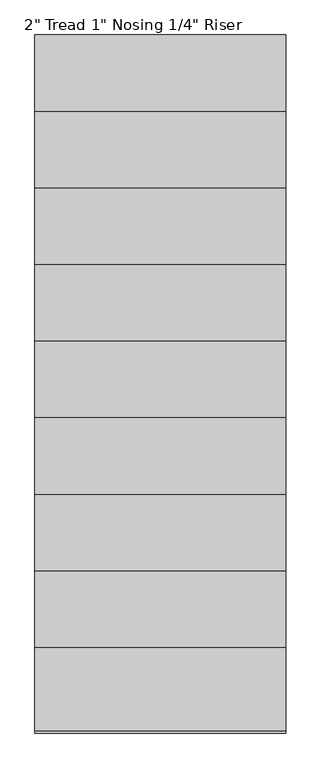
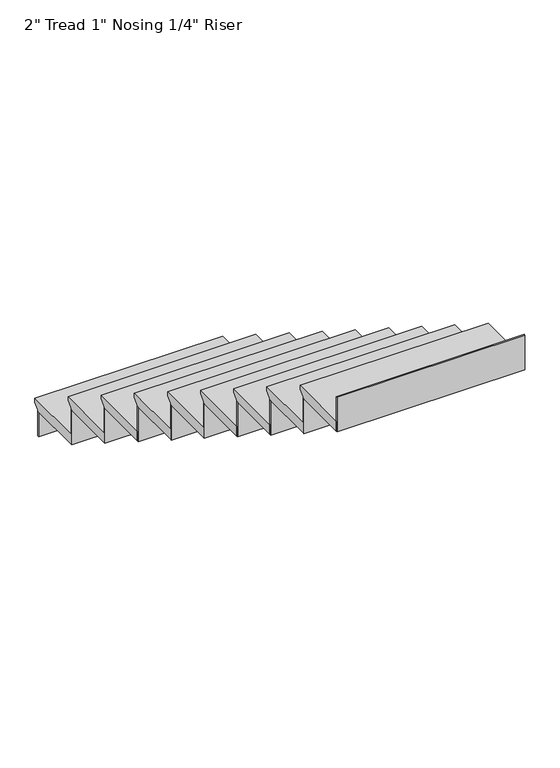
"""IFC4 building model written with IfcOpenShell, lengths in millimetres: stair flight geometry."""

from ifc_helpers import new_model, si_unit, origin, place, context, project, spatial, faceted_brep, source, transform, mapped, element, save


def stair_flight_61f47217(model_context):
    return source(origin(), model_context, "Body", "Brep", [
        faceted_brep([(-3651.3993763, -1023.9064015, 768.35), (-3651.3993763, -1023.9064015, 787.4), (-2736.9993763, -1023.9064015, 787.4), (-2736.9993763, -1023.9064015, 768.35), (-3651.3993763, -1049.3064015, 742.95), (-2736.9993763, -1049.3064015, 742.95), (-3651.3993763, -1328.7064015, 787.4), (-2736.9993763, -1328.7064015, 787.4), (-2736.9993763, -1049.3064015, 736.6), (-2736.9993763, -1328.7064015, 736.6), (-3651.3993763, -1328.7064015, 736.6), (-3651.3993763, -1049.3064015, 736.6)], [[[0, 1, 2, 3]], [[4, 0, 3, 5]], [[2, 1, 6, 7]], [[8, 9, 10, 11]], [[2, 7, 9, 8, 5, 3]], [[8, 11, 4, 5]], [[6, 1, 0, 4, 11, 10]], [[7, 6, 10, 9]]]),
        faceted_brep([(-3651.3993763, -1049.3064015, 736.6), (-3651.3993763, -1049.3064015, 609.6), (-3651.3993763, -1055.6564015, 609.6), (-3651.3993763, -1055.6564015, 736.6), (-2736.9993763, -1049.3064015, 736.6), (-2736.9993763, -1055.6564015, 736.6), (-2736.9993763, -1055.6564015, 609.6), (-2736.9993763, -1049.3064015, 609.6)], [[[0, 1, 2, 3]], [[4, 5, 6, 7]], [[1, 0, 4, 7]], [[2, 1, 7, 6]], [[3, 2, 6, 5]], [[0, 3, 5, 4]]]),
        faceted_brep([(-3651.3993763, -1328.7064015, 914.4), (-3651.3993763, -1328.7064015, 736.6), (-3651.3993763, -1335.0564015, 736.6), (-3651.3993763, -1335.0564015, 914.4), (-2736.9993763, -1328.7064015, 914.4), (-2736.9993763, -1335.0564015, 914.4), (-2736.9993763, -1335.0564015, 736.6), (-2736.9993763, -1328.7064015, 736.6)], [[[0, 1, 2, 3]], [[4, 5, 6, 7]], [[1, 0, 4, 7]], [[2, 1, 7, 6]], [[3, 2, 6, 5]], [[0, 3, 5, 4]]]),
        faceted_brep([(-2736.9993763, -1303.3064015, 965.2), (-3651.3993763, -1303.3064015, 965.2), (-3651.3993763, -1608.1064015, 965.2), (-2736.9993763, -1608.1064015, 965.2), (-2736.9993763, -1328.7064015, 914.4), (-2736.9993763, -1608.1064015, 914.4), (-3651.3993763, -1608.1064015, 914.4), (-3651.3993763, -1328.7064015, 914.4), (-2736.9993763, -1328.7064015, 920.75), (-2736.9993763, -1303.3064015, 946.15), (-3651.3993763, -1328.7064015, 920.75), (-3651.3993763, -1303.3064015, 946.15)], [[[0, 1, 2, 3]], [[4, 5, 6, 7]], [[0, 3, 5, 4, 8, 9]], [[4, 7, 10, 8]], [[2, 1, 11, 10, 7, 6]], [[3, 2, 6, 5]], [[11, 1, 0, 9]], [[10, 11, 9, 8]]]),
        faceted_brep([(-3651.3993763, -1608.1064015, 1092.2), (-3651.3993763, -1608.1064015, 914.4), (-3651.3993763, -1614.4564015, 914.4), (-3651.3993763, -1614.4564015, 1092.2), (-2736.9993763, -1608.1064015, 1092.2), (-2736.9993763, -1614.4564015, 1092.2), (-2736.9993763, -1614.4564015, 914.4), (-2736.9993763, -1608.1064015, 914.4)], [[[0, 1, 2, 3]], [[4, 5, 6, 7]], [[1, 0, 4, 7]], [[2, 1, 7, 6]], [[3, 2, 6, 5]], [[0, 3, 5, 4]]]),
        faceted_brep([(-2736.9993763, -1582.7064015, 1143.0), (-3651.3993763, -1582.7064015, 1143.0), (-3651.3993763, -1887.5064015, 1143.0), (-2736.9993763, -1887.5064015, 1143.0), (-2736.9993763, -1608.1064015, 1092.2), (-2736.9993763, -1887.5064015, 1092.2), (-3651.3993763, -1887.5064015, 1092.2), (-3651.3993763, -1608.1064015, 1092.2), (-2736.9993763, -1608.1064015, 1098.55), (-2736.9993763, -1582.7064015, 1123.95), (-3651.3993763, -1608.1064015, 1098.55), (-3651.3993763, -1582.7064015, 1123.95)], [[[0, 1, 2, 3]], [[4, 5, 6, 7]], [[0, 3, 5, 4, 8, 9]], [[4, 7, 10, 8]], [[2, 1, 11, 10, 7, 6]], [[3, 2, 6, 5]], [[11, 1, 0, 9]], [[10, 11, 9, 8]]]),
        faceted_brep([(-3651.3993763, -1887.5064015, 1270.0), (-3651.3993763, -1887.5064015, 1092.2), (-3651.3993763, -1893.8564015, 1092.2), (-3651.3993763, -1893.8564015, 1270.0), (-2736.9993763, -1887.5064015, 1270.0), (-2736.9993763, -1893.8564015, 1270.0), (-2736.9993763, -1893.8564015, 1092.2), (-2736.9993763, -1887.5064015, 1092.2)], [[[0, 1, 2, 3]], [[4, 5, 6, 7]], [[1, 0, 4, 7]], [[2, 1, 7, 6]], [[3, 2, 6, 5]], [[0, 3, 5, 4]]]),
        faceted_brep([(-2736.9993763, -1862.1064015, 1320.8), (-3651.3993763, -1862.1064015, 1320.8), (-3651.3993763, -2166.9064015, 1320.8), (-2736.9993763, -2166.9064015, 1320.8), (-2736.9993763, -1887.5064015, 1270.0), (-2736.9993763, -2166.9064015, 1270.0), (-3651.3993763, -2166.9064015, 1270.0), (-3651.3993763, -1887.5064015, 1270.0), (-2736.9993763, -1887.5064015, 1276.35), (-2736.9993763, -1862.1064015, 1301.75), (-3651.3993763, -1887.5064015, 1276.35), (-3651.3993763, -1862.1064015, 1301.75)], [[[0, 1, 2, 3]], [[4, 5, 6, 7]], [[0, 3, 5, 4, 8, 9]], [[4, 7, 10, 8]], [[2, 1, 11, 10, 7, 6]], [[3, 2, 6, 5]], [[11, 1, 0, 9]], [[10, 11, 9, 8]]]),
        faceted_brep([(-3651.3993763, -2166.9064015, 1447.8), (-3651.3993763, -2166.9064015, 1270.0), (-3651.3993763, -2173.2564015, 1270.0), (-3651.3993763, -2173.2564015, 1447.8), (-2736.9993763, -2166.9064015, 1447.8), (-2736.9993763, -2173.2564015, 1447.8), (-2736.9993763, -2173.2564015, 1270.0), (-2736.9993763, -2166.9064015, 1270.0)], [[[0, 1, 2, 3]], [[4, 5, 6, 7]], [[1, 0, 4, 7]], [[2, 1, 7, 6]], [[3, 2, 6, 5]], [[0, 3, 5, 4]]]),
        faceted_brep([(-2736.9993763, -2141.5064015, 1498.6), (-3651.3993763, -2141.5064015, 1498.6), (-3651.3993763, -2446.3064015, 1498.6), (-2736.9993763, -2446.3064015, 1498.6), (-2736.9993763, -2166.9064015, 1447.8), (-2736.9993763, -2446.3064015, 1447.8), (-3651.3993763, -2446.3064015, 1447.8), (-3651.3993763, -2166.9064015, 1447.8), (-2736.9993763, -2166.9064015, 1454.15), (-2736.9993763, -2141.5064015, 1479.55), (-3651.3993763, -2166.9064015, 1454.15), (-3651.3993763, -2141.5064015, 1479.55)], [[[0, 1, 2, 3]], [[4, 5, 6, 7]], [[0, 3, 5, 4, 8, 9]], [[4, 7, 10, 8]], [[2, 1, 11, 10, 7, 6]], [[3, 2, 6, 5]], [[11, 1, 0, 9]], [[10, 11, 9, 8]]]),
        faceted_brep([(-3651.3993763, -2446.3064015, 1625.6), (-3651.3993763, -2446.3064015, 1447.8), (-3651.3993763, -2452.6564015, 1447.8), (-3651.3993763, -2452.6564015, 1625.6), (-2736.9993763, -2446.3064015, 1625.6), (-2736.9993763, -2452.6564015, 1625.6), (-2736.9993763, -2452.6564015, 1447.8), (-2736.9993763, -2446.3064015, 1447.8)], [[[0, 1, 2, 3]], [[4, 5, 6, 7]], [[1, 0, 4, 7]], [[2, 1, 7, 6]], [[3, 2, 6, 5]], [[0, 3, 5, 4]]]),
        faceted_brep([(-2736.9993763, -2420.9064015, 1676.4), (-3651.3993763, -2420.9064015, 1676.4), (-3651.3993763, -2725.7064015, 1676.4), (-2736.9993763, -2725.7064015, 1676.4), (-2736.9993763, -2446.3064015, 1625.6), (-2736.9993763, -2725.7064015, 1625.6), (-3651.3993763, -2725.7064015, 1625.6), (-3651.3993763, -2446.3064015, 1625.6), (-2736.9993763, -2446.3064015, 1631.95), (-2736.9993763, -2420.9064015, 1657.35), (-3651.3993763, -2446.3064015, 1631.95), (-3651.3993763, -2420.9064015, 1657.35)], [[[0, 1, 2, 3]], [[4, 5, 6, 7]], [[0, 3, 5, 4, 8, 9]], [[4, 7, 10, 8]], [[2, 1, 11, 10, 7, 6]], [[3, 2, 6, 5]], [[11, 1, 0, 9]], [[10, 11, 9, 8]]]),
        faceted_brep([(-3651.3993763, -2725.7064015, 1803.4), (-3651.3993763, -2725.7064015, 1625.6), (-3651.3993763, -2732.0564015, 1625.6), (-3651.3993763, -2732.0564015, 1803.4), (-2736.9993763, -2725.7064015, 1803.4), (-2736.9993763, -2732.0564015, 1803.4), (-2736.9993763, -2732.0564015, 1625.6), (-2736.9993763, -2725.7064015, 1625.6)], [[[0, 1, 2, 3]], [[4, 5, 6, 7]], [[1, 0, 4, 7]], [[2, 1, 7, 6]], [[3, 2, 6, 5]], [[0, 3, 5, 4]]]),
        faceted_brep([(-2736.9993763, -2700.3064015, 1854.2), (-3651.3993763, -2700.3064015, 1854.2), (-3651.3993763, -3005.1064015, 1854.2), (-2736.9993763, -3005.1064015, 1854.2), (-2736.9993763, -2725.7064015, 1803.4), (-2736.9993763, -3005.1064015, 1803.4), (-3651.3993763, -3005.1064015, 1803.4), (-3651.3993763, -2725.7064015, 1803.4), (-2736.9993763, -2725.7064015, 1809.75), (-2736.9993763, -2700.3064015, 1835.15), (-3651.3993763, -2725.7064015, 1809.75), (-3651.3993763, -2700.3064015, 1835.15)], [[[0, 1, 2, 3]], [[4, 5, 6, 7]], [[0, 3, 5, 4, 8, 9]], [[4, 7, 10, 8]], [[2, 1, 11, 10, 7, 6]], [[3, 2, 6, 5]], [[11, 1, 0, 9]], [[10, 11, 9, 8]]]),
        faceted_brep([(-3651.3993763, -3005.1064015, 1981.2), (-3651.3993763, -3005.1064015, 1803.4), (-3651.3993763, -3011.4564015, 1803.4), (-3651.3993763, -3011.4564015, 1981.2), (-2736.9993763, -3005.1064015, 1981.2), (-2736.9993763, -3011.4564015, 1981.2), (-2736.9993763, -3011.4564015, 1803.4), (-2736.9993763, -3005.1064015, 1803.4)], [[[0, 1, 2, 3]], [[4, 5, 6, 7]], [[1, 0, 4, 7]], [[2, 1, 7, 6]], [[3, 2, 6, 5]], [[0, 3, 5, 4]]]),
        faceted_brep([(-2736.9993763, -2979.7064015, 2032.0), (-3651.3993763, -2979.7064015, 2032.0), (-3651.3993763, -3284.5064015, 2032.0), (-2736.9993763, -3284.5064015, 2032.0), (-2736.9993763, -3005.1064015, 1981.2), (-2736.9993763, -3284.5064015, 1981.2), (-3651.3993763, -3284.5064015, 1981.2), (-3651.3993763, -3005.1064015, 1981.2), (-2736.9993763, -3005.1064015, 1987.55), (-2736.9993763, -2979.7064015, 2012.95), (-3651.3993763, -3005.1064015, 1987.55), (-3651.3993763, -2979.7064015, 2012.95)], [[[0, 1, 2, 3]], [[4, 5, 6, 7]], [[0, 3, 5, 4, 8, 9]], [[4, 7, 10, 8]], [[2, 1, 11, 10, 7, 6]], [[3, 2, 6, 5]], [[11, 1, 0, 9]], [[10, 11, 9, 8]]]),
        faceted_brep([(-3651.3993763, -3563.9064015, 2336.8), (-3651.3993763, -3563.9064015, 2159.0), (-3651.3993763, -3570.2564015, 2159.0), (-3651.3993763, -3570.2564015, 2336.8), (-2736.9993763, -3563.9064015, 2336.8), (-2736.9993763, -3570.2564015, 2336.8), (-2736.9993763, -3570.2564015, 2159.0), (-2736.9993763, -3563.9064015, 2159.0)], [[[0, 1, 2, 3]], [[4, 5, 6, 7]], [[1, 0, 4, 7]], [[2, 1, 7, 6]], [[3, 2, 6, 5]], [[0, 3, 5, 4]]]),
        faceted_brep([(-3651.3993763, -3284.5064015, 2159.0), (-3651.3993763, -3284.5064015, 1981.2), (-3651.3993763, -3290.8564015, 1981.2), (-3651.3993763, -3290.8564015, 2159.0), (-2736.9993763, -3284.5064015, 2159.0), (-2736.9993763, -3290.8564015, 2159.0), (-2736.9993763, -3290.8564015, 1981.2), (-2736.9993763, -3284.5064015, 1981.2)], [[[0, 1, 2, 3]], [[4, 5, 6, 7]], [[1, 0, 4, 7]], [[2, 1, 7, 6]], [[3, 2, 6, 5]], [[0, 3, 5, 4]]]),
        faceted_brep([(-2736.9993763, -3563.9064015, 2209.8), (-2736.9993763, -3538.5064015, 2209.8), (-2736.9993763, -3259.1064015, 2209.8), (-3651.3993763, -3259.1064015, 2209.8), (-3651.3993763, -3563.9064015, 2209.8), (-2736.9993763, -3538.5064015, 2159.0), (-2736.9993763, -3563.9064015, 2159.0), (-3651.3993763, -3563.9064015, 2159.0), (-3651.3993763, -3284.5064015, 2159.0), (-2736.9993763, -3284.5064015, 2159.0), (-2736.9993763, -3284.5064015, 2165.35), (-2736.9993763, -3259.1064015, 2190.75), (-3651.3993763, -3284.5064015, 2165.35), (-3651.3993763, -3259.1064015, 2190.75)], [[[0, 1, 2, 3, 4]], [[5, 6, 7, 8, 9]], [[1, 0, 6, 5]], [[2, 1, 5, 9, 10, 11]], [[9, 8, 12, 10]], [[4, 3, 13, 12, 8, 7]], [[0, 4, 7, 6]], [[13, 3, 2, 11]], [[12, 13, 11, 10]]]),
    ])


if __name__ == "__main__":
    model = new_model("IFC4")
    model_context = context("Model", 3, world=origin())
    ifc_project = project(units=[si_unit("LENGTHUNIT", "METRE", prefix="MILLI")], contexts=[model_context])
    site = spatial("IfcSite", under=ifc_project)
    building = spatial("IfcBuilding", under=site)
    placement = place(None, origin())
    stair_flight_shape = stair_flight_61f47217(model_context)
    element("IfcStairFlight", 1, ObjectType="2\" Tread 1\" Nosing 1/4\" Riser", at=placement, inside=building, context=model_context, shape_type="MappedRepresentation", body=[
        mapped(stair_flight_shape, transform((0.0, 0.0, 0.0), x_axis=(1.0, 0.0, 0.0), y_axis=(0.0, 1.0, 0.0), z_axis=(0.0, 0.0, 1.0))),
    ])
    save(model, "model.ifc")
